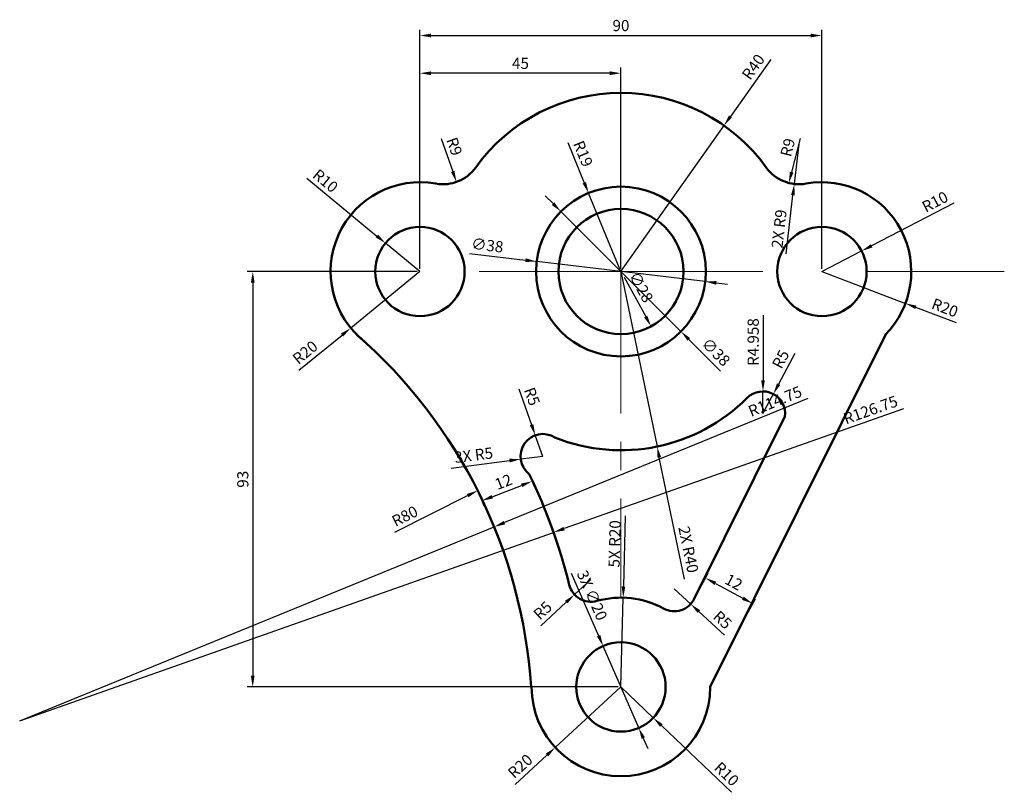
# Model space of a CAD drawing. Units: millimetres. Extents: x -135 to 86, y -117 to 56.
import ezdxf

# ---------------------------------------------------------------- set-up
doc = ezdxf.new("R2010")
doc.units = ezdxf.units.MM
doc.linetypes.add('CENTER', pattern=[50.8, 31.75, -6.35, 6.35, -6.35])
for name, color, linetype, lineweight in [('M-CNTR', 4, 'CENTER', 18), ('M-DIMS', 2, 'Continuous', 25), ('M-OUTL', 7, 'Continuous', 50)]:
    doc.layers.add(name, color=color, linetype=linetype, lineweight=lineweight)
doc.styles.get("Standard").update_dxf_attribs({"font": 'arial.ttf'})
doc.dimstyles.new('ISO-25', dxfattribs={"dimtxt": 2.5, "dimasz": 2.5, "dimexe": 1.25, "dimexo": 0.625, "dimtad": 1, "dimtxsty": 'Standard', "dimcen": 2.5, "dimadec": 0, "dimazin": 0, "dimtfac": 1, "dimtmove": 0, "dimatfit": 3, "dimfxl": 1, "dimarcsym": 0})

# ---------------------------------------------------------------- blocks, each defined once
blk = doc.blocks.new('*D1')
at = {"layer": 'Defpoints', "color": 0, "transparency": 16777216}
for p in [(0, -93), (-14.72, -106.54)]:
    blk.add_point(p, dxfattribs=at)
at = {"layer": 'M-DIMS', "color": 0, "lineweight": -2, "transparency": 16777216}
for p, q in [((0, -93), (-14.72, -106.54)), ((-23.71, -114.81), (-16.56, -108.23))]:
    blk.add_line(p, q, dxfattribs=at)
at = {"layer": 'M-DIMS', "color": 0, "transparency": 16777216}
blk.add_solid([(-16.84, -107.92), (-16.28, -108.54), (-14.72, -106.54)], dxfattribs=at)
at = {"layer": 'M-DIMS', "color": 0, "transparency": 16777216, "insert": (-22.34, -110.96), "char_height": 2.5, "attachment_point": 5, "rotation": 42.6003}
blk.add_mtext('R20', dxfattribs=at)
blk = doc.blocks.new('*D2')
at = {"layer": 'Defpoints', "color": 0, "transparency": 16777216}
for p in [(45, 0), (63.69, -7.12)]:
    blk.add_point(p, dxfattribs=at)
at = {"layer": 'M-DIMS', "color": 0, "lineweight": -2, "transparency": 16777216}
for p, q in [((45, 0), (63.69, -7.12)), ((75.1, -11.48), (66.02, -8.02))]:
    blk.add_line(p, q, dxfattribs=at)
at = {"layer": 'M-DIMS', "color": 0, "transparency": 16777216}
blk.add_solid([(66.17, -7.63), (65.88, -8.4), (63.69, -7.12)], dxfattribs=at)
at = {"layer": 'M-DIMS', "color": 0, "transparency": 16777216, "insert": (72.41, -8.41), "char_height": 2.5, "attachment_point": 5, "rotation": 339.13}
blk.add_mtext('R20', dxfattribs=at)
blk = doc.blocks.new('*D3')
at = {"layer": 'Defpoints', "color": 0, "transparency": 16777216}
for p in [(-45, 0), (-60.5, -12.64)]:
    blk.add_point(p, dxfattribs=at)
at = {"layer": 'M-DIMS', "color": 0, "lineweight": -2, "transparency": 16777216}
for p, q in [((-45, 0), (-60.5, -12.64)), ((-72.11, -22.1), (-62.44, -14.22))]:
    blk.add_line(p, q, dxfattribs=at)
at = {"layer": 'M-DIMS', "color": 0, "transparency": 16777216}
blk.add_solid([(-62.7, -13.89), (-62.18, -14.54), (-60.5, -12.64)], dxfattribs=at)
at = {"layer": 'M-DIMS', "color": 0, "transparency": 16777216, "insert": (-70.51, -18.35), "char_height": 2.5, "attachment_point": 5, "rotation": 39.1885}
blk.add_mtext('R20', dxfattribs=at)
blk = doc.blocks.new('*D4')
at = {"layer": 'Defpoints', "color": 0, "transparency": 16777216}
for p in [(-52.72, 6.36), (-45, 0)]:
    blk.add_point(p, dxfattribs=at)
at = {"layer": 'M-DIMS', "color": 0, "lineweight": -2, "transparency": 16777216}
for p, q in [((-70.35, 20.88), (-54.65, 7.95)), ((-45, 0), (-52.72, 6.36))]:
    blk.add_line(p, q, dxfattribs=at)
at = {"layer": 'M-DIMS', "color": 0, "transparency": 16777216}
blk.add_solid([(-54.38, 8.27), (-54.91, 7.63), (-52.72, 6.36)], dxfattribs=at)
at = {"layer": 'M-DIMS', "color": 0, "transparency": 16777216, "insert": (-66.36, 20.05), "char_height": 2.5, "attachment_point": 5, "rotation": 320.5239}
blk.add_mtext('R10', dxfattribs=at)
blk = doc.blocks.new('*D5')
at = {"layer": 'Defpoints', "color": 0, "transparency": 16777216}
for p in [(53.88, 4.6), (45, 0)]:
    blk.add_point(p, dxfattribs=at)
at = {"layer": 'M-DIMS', "color": 0, "lineweight": -2, "transparency": 16777216}
for p, q in [((74.53, 15.3), (56.1, 5.75)), ((45, 0), (53.88, 4.6))]:
    blk.add_line(p, q, dxfattribs=at)
at = {"layer": 'M-DIMS', "color": 0, "transparency": 16777216}
blk.add_solid([(55.91, 6.12), (56.29, 5.38), (53.88, 4.6)], dxfattribs=at)
at = {"layer": 'M-DIMS', "color": 0, "transparency": 16777216, "insert": (70.46, 15.33), "char_height": 2.5, "attachment_point": 5, "rotation": 27.3837}
blk.add_mtext('R10', dxfattribs=at)
blk = doc.blocks.new('*D6')
at = {"layer": 'Defpoints', "color": 0, "transparency": 16777216}
for p in [(0, -93), (7.24, -99.9)]:
    blk.add_point(p, dxfattribs=at)
at = {"layer": 'M-DIMS', "color": 0, "lineweight": -2, "transparency": 16777216}
for p, q in [((0, -93), (7.24, -99.9)), ((24.73, -116.58), (9.05, -101.63))]:
    blk.add_line(p, q, dxfattribs=at)
at = {"layer": 'M-DIMS', "color": 0, "transparency": 16777216}
blk.add_solid([(9.33, -101.32), (8.76, -101.93), (7.24, -99.9)], dxfattribs=at)
at = {"layer": 'M-DIMS', "color": 0, "transparency": 16777216, "insert": (23.43, -112.71), "char_height": 2.5, "attachment_point": 5, "rotation": 316.3688}
blk.add_mtext('R10', dxfattribs=at)
blk = doc.blocks.new('*D7')
at = {"layer": 'Defpoints', "color": 0, "transparency": 16777216}
for p in [(23.07, 32.68), (0, 0)]:
    blk.add_point(p, dxfattribs=at)
at = {"layer": 'M-DIMS', "color": 0, "lineweight": -2, "transparency": 16777216}
for p, q in [((33.52, 47.48), (24.51, 34.72)), ((0, 0), (23.07, 32.68))]:
    blk.add_line(p, q, dxfattribs=at)
at = {"layer": 'M-DIMS', "color": 0, "transparency": 16777216}
blk.add_solid([(24.17, 34.96), (24.85, 34.48), (23.07, 32.68)], dxfattribs=at)
at = {"layer": 'M-DIMS', "color": 0, "transparency": 16777216, "insert": (29.89, 45.63), "char_height": 2.5, "attachment_point": 5, "rotation": 54.7774}
blk.add_mtext('R40', dxfattribs=at)
blk = doc.blocks.new('*D8')
at = {"layer": 'Defpoints', "color": 0, "transparency": 16777216}
for p in [(-6.74, 12.27), (6.74, -12.27)]:
    blk.add_point(p, dxfattribs=at)
at = {"layer": 'M-DIMS', "color": 0, "lineweight": -2, "transparency": 16777216}
blk.add_line((0.7, -1.27), (5.54, -10.08), dxfattribs=at)
at = {"layer": 'M-DIMS', "color": 0, "transparency": 16777216}
blk.add_solid([(5.9, -9.88), (5.17, -10.28), (6.74, -12.27)], dxfattribs=at)
at = {"layer": 'M-DIMS', "color": 0, "transparency": 16777216, "insert": (4.24, -3.63), "char_height": 2.5, "attachment_point": 5, "rotation": 298.7887}
blk.add_mtext('∅28', dxfattribs=at)
blk = doc.blocks.new('*D9')
at = {"layer": 'Defpoints', "color": 0, "transparency": 16777216}
for p in [(-13.44, 13.43), (13.44, -13.43)]:
    blk.add_point(p, dxfattribs=at)
at = {"layer": 'M-DIMS', "color": 0, "lineweight": -2, "transparency": 16777216}
for p, q in [((-15.21, 15.2), (-16.98, 16.96)), ((-13.44, 13.43), (13.44, -13.43)), ((22.32, -22.3), (15.21, -15.2))]:
    blk.add_line(p, q, dxfattribs=at)
at = {"layer": 'M-DIMS', "color": 0, "transparency": 16777216}
for points in [[(-14.92, 15.49), (-15.5, 14.9), (-13.44, 13.43)], [(15.5, -14.9), (14.92, -15.49), (13.44, -13.43)]]:
    blk.add_solid(points, dxfattribs=at)
at = {"layer": 'M-DIMS', "color": 0, "transparency": 16777216, "insert": (21.04, -18.24), "char_height": 2.5, "attachment_point": 5, "rotation": 315.0277}
blk.add_mtext('∅38', dxfattribs=at)
blk = doc.blocks.new('*D10')
at = {"layer": 'Defpoints', "color": 0, "transparency": 16777216}
for p in [(39.83, 28.54), (37.59, 19.82)]:
    blk.add_point(p, dxfattribs=at)
at = {"layer": 'M-DIMS', "color": 0, "lineweight": -2, "transparency": 16777216}
blk.add_line((40.15, 29.78), (38.21, 22.24), dxfattribs=at)
at = {"layer": 'M-DIMS', "color": 0, "transparency": 16777216}
blk.add_solid([(37.81, 22.35), (38.62, 22.14), (37.59, 19.82)], dxfattribs=at)
at = {"layer": 'M-DIMS', "color": 0, "transparency": 16777216, "insert": (37.65, 27.7), "char_height": 2.5, "attachment_point": 5, "rotation": 75.5659}
blk.add_mtext('R9', dxfattribs=at)
blk = doc.blocks.new('*D11')
at = {"layer": 'Defpoints', "color": 0, "transparency": 16777216}
for p in [(-39.83, 28.54), (-36.84, 20.05)]:
    blk.add_point(p, dxfattribs=at)
at = {"layer": 'M-DIMS', "color": 0, "lineweight": -2, "transparency": 16777216}
blk.add_line((-40.26, 29.75), (-37.67, 22.41), dxfattribs=at)
at = {"layer": 'M-DIMS', "color": 0, "transparency": 16777216}
blk.add_solid([(-37.28, 22.55), (-38.06, 22.27), (-36.84, 20.05)], dxfattribs=at)
at = {"layer": 'M-DIMS', "color": 0, "transparency": 16777216, "insert": (-37.59, 27.89), "char_height": 2.5, "attachment_point": 5, "rotation": 289.4447}
blk.add_mtext('R9', dxfattribs=at)
blk = doc.blocks.new('*D12')
at = {"layer": 'Defpoints', "color": 0, "transparency": 16777216}
for p in [(-7.25, 17.56), (0, 0)]:
    blk.add_point(p, dxfattribs=at)
at = {"layer": 'M-DIMS', "color": 0, "lineweight": -2, "transparency": 16777216}
for p, q in [((-11.91, 28.87), (-8.2, 19.87)), ((0, 0), (-7.25, 17.56))]:
    blk.add_line(p, q, dxfattribs=at)
at = {"layer": 'M-DIMS', "color": 0, "transparency": 16777216}
blk.add_solid([(-7.82, 20.03), (-8.59, 19.72), (-7.25, 17.56)], dxfattribs=at)
at = {"layer": 'M-DIMS', "color": 0, "transparency": 16777216, "insert": (-8.78, 26.25), "char_height": 2.5, "attachment_point": 5, "rotation": 292.423}
blk.add_mtext('R19', dxfattribs=at)
blk = doc.blocks.new('*D13')
at = {"layer": 'Defpoints', "color": 0, "transparency": 16777216}
for p in [(-45, 44.39), (0, 0), (-45, 0)]:
    blk.add_point(p, dxfattribs=at)
at = {"layer": 'M-DIMS', "color": 0, "lineweight": -2, "transparency": 16777216}
for p, q in [((-45, 0.62), (-45, 45.64)), ((-2.5, 44.39), (-42.5, 44.39)), ((0, 0.62), (0, 45.64))]:
    blk.add_line(p, q, dxfattribs=at)
at = {"layer": 'M-DIMS', "color": 0, "transparency": 16777216}
for points in [[(-42.5, 44.81), (-42.5, 43.97), (-45, 44.39)], [(-2.5, 44.81), (-2.5, 43.97), (0, 44.39)]]:
    blk.add_solid(points, dxfattribs=at)
at = {"layer": 'M-DIMS', "color": 0, "transparency": 16777216, "insert": (-22.5, 46.29), "char_height": 2.5, "attachment_point": 5}
blk.add_mtext('45', dxfattribs=at)
blk = doc.blocks.new('*D14')
at = {"layer": 'Defpoints', "color": 0, "transparency": 16777216}
for p in [(45, 52.83), (45, 0), (-45, 0)]:
    blk.add_point(p, dxfattribs=at)
at = {"layer": 'M-DIMS', "color": 0, "lineweight": -2, "transparency": 16777216}
for p, q in [((-45, 0.62), (-45, 54.08)), ((45, 0.62), (45, 54.08)), ((-42.5, 52.83), (42.5, 52.83))]:
    blk.add_line(p, q, dxfattribs=at)
at = {"layer": 'M-DIMS', "color": 0, "transparency": 16777216}
for points in [[(-42.5, 53.25), (-42.5, 52.42), (-45, 52.83)], [(42.5, 53.25), (42.5, 52.42), (45, 52.83)]]:
    blk.add_solid(points, dxfattribs=at)
at = {"layer": 'M-DIMS', "color": 0, "transparency": 16777216, "insert": (0, 54.74), "char_height": 2.5, "attachment_point": 5}
blk.add_mtext('90', dxfattribs=at)
blk = doc.blocks.new('*D15')
at = {"layer": 'Defpoints', "color": 0, "transparency": 16777216}
for p in [(16.41, -73.26), (29.49, -74.33), (26.97, -78.98)]:
    blk.add_point(p, dxfattribs=at)
at = {"layer": 'M-DIMS', "color": 0, "lineweight": -2, "transparency": 16777216}
for p, q in [((16.71, -72.71), (19.53, -67.51)), ((21.13, -69.8), (27.29, -73.13)), ((27.27, -78.43), (30.09, -73.23))]:
    blk.add_line(p, q, dxfattribs=at)
at = {"layer": 'M-DIMS', "color": 0, "transparency": 16777216}
for points in [[(21.33, -69.43), (20.93, -70.17), (18.93, -68.61)], [(27.49, -72.77), (27.1, -73.5), (29.49, -74.33)]]:
    blk.add_solid(points, dxfattribs=at)
at = {"layer": 'M-DIMS', "color": 0, "transparency": 16777216, "insert": (25.11, -69.81), "char_height": 2.5, "attachment_point": 5, "rotation": 331.5726}
blk.add_mtext('12', dxfattribs=at)
blk = doc.blocks.new('*D16')
at = {"layer": 'Defpoints', "color": 0, "transparency": 16777216}
for p in [(-20.54, -45.33), (-19.9, -46.96), (-31.77, -49.68)]:
    blk.add_point(p, dxfattribs=at)
at = {"layer": 'M-DIMS', "color": 0, "lineweight": -2, "transparency": 16777216}
for p, q in [((-20.31, -45.92), (-19.45, -48.13)), ((-28.81, -50.41), (-22.24, -47.87)), ((-31.54, -50.26), (-30.69, -52.48))]:
    blk.add_line(p, q, dxfattribs=at)
at = {"layer": 'M-DIMS', "color": 0, "transparency": 16777216}
for points in [[(-22.39, -47.48), (-22.09, -48.25), (-19.9, -46.96)], [(-28.96, -50.02), (-28.66, -50.8), (-31.14, -51.31)]]:
    blk.add_solid(points, dxfattribs=at)
at = {"layer": 'M-DIMS', "color": 0, "transparency": 16777216, "insert": (-26.2, -47.38), "char_height": 2.5, "attachment_point": 5, "rotation": 21.1544}
blk.add_mtext('12', dxfattribs=at)
blk = doc.blocks.new('*D17')
at = {"layer": 'Defpoints', "color": 0, "transparency": 16777216}
for p in [(-32.09, -49.04), (-134.61, -100.59)]:
    blk.add_point(p, dxfattribs=at)
at = {"layer": 'M-DIMS', "color": 0, "lineweight": -2, "transparency": 16777216}
blk.add_line((-50.61, -58.36), (-34.32, -50.17), dxfattribs=at)
at = {"layer": 'M-DIMS', "color": 0, "transparency": 16777216}
blk.add_solid([(-34.51, -49.79), (-34.13, -50.54), (-32.09, -49.04)], dxfattribs=at)
at = {"layer": 'M-DIMS', "color": 0, "transparency": 16777216, "insert": (-48.24, -55.04), "char_height": 2.5, "attachment_point": 5, "rotation": 26.6892}
blk.add_mtext('R80', dxfattribs=at)
blk = doc.blocks.new('*D18')
at = {"layer": 'Defpoints', "color": 0, "transparency": 16777216}
for p in [(-45, 0), (-82.44, -93), (0, -93)]:
    blk.add_point(p, dxfattribs=at)
at = {"layer": 'M-DIMS', "color": 0, "lineweight": -2, "transparency": 16777216}
for p, q in [((-45.63, 0), (-83.69, 0)), ((-82.44, -2.5), (-82.44, -90.5)), ((-0.63, -93), (-83.69, -93))]:
    blk.add_line(p, q, dxfattribs=at)
at = {"layer": 'M-DIMS', "color": 0, "transparency": 16777216}
for points in [[(-82.85, -2.5), (-82.02, -2.5), (-82.44, 0)], [(-82.85, -90.5), (-82.02, -90.5), (-82.44, -93)]]:
    blk.add_solid(points, dxfattribs=at)
at = {"layer": 'M-DIMS', "color": 0, "transparency": 16777216, "insert": (-84.34, -46.5), "char_height": 2.5, "attachment_point": 5, "rotation": 90}
blk.add_mtext('93', dxfattribs=at)
blk = doc.blocks.new('*D19')
at = {"layer": 'Defpoints', "color": 0, "transparency": 16777216}
for p in [(-19.17, -36.66), (-17.49, -41.37)]:
    blk.add_point(p, dxfattribs=at)
at = {"layer": 'M-DIMS', "color": 0, "lineweight": -2, "transparency": 16777216}
for p, q in [((-22.89, -26.22), (-20.01, -34.3)), ((-17.49, -41.37), (-19.17, -36.66))]:
    blk.add_line(p, q, dxfattribs=at)
at = {"layer": 'M-DIMS', "color": 0, "transparency": 16777216}
blk.add_solid([(-19.62, -34.16), (-20.4, -34.44), (-19.17, -36.66)], dxfattribs=at)
at = {"layer": 'M-DIMS', "color": 0, "transparency": 16777216, "insert": (-20.21, -28.08), "char_height": 2.5, "attachment_point": 5, "rotation": 289.6107}
blk.add_mtext('R5', dxfattribs=at)
blk = doc.blocks.new('*D20')
at = {"layer": 'Defpoints', "color": 0, "transparency": 16777216}
for p in [(34.12, -27.41), (31.79, -31.79)]:
    blk.add_point(p, dxfattribs=at)
at = {"layer": 'M-DIMS', "color": 0, "lineweight": -2, "transparency": 16777216}
for p, q in [((38.96, -18.32), (35.29, -25.21)), ((31.79, -31.79), (34.12, -27.41))]:
    blk.add_line(p, q, dxfattribs=at)
at = {"layer": 'M-DIMS', "color": 0, "transparency": 16777216}
blk.add_solid([(34.93, -25.01), (35.66, -25.4), (34.12, -27.41)], dxfattribs=at)
at = {"layer": 'M-DIMS', "color": 0, "transparency": 16777216, "insert": (36.04, -19.77), "char_height": 2.5, "attachment_point": 5, "rotation": 61.9797}
blk.add_mtext('R5', dxfattribs=at)
blk = doc.blocks.new('*D21')
at = {"layer": 'Defpoints', "color": 0, "transparency": 16777216}
for p in [(11.94, -71.03), (15.61, -74.43)]:
    blk.add_point(p, dxfattribs=at)
at = {"layer": 'M-DIMS', "color": 0, "lineweight": -2, "transparency": 16777216}
for p, q in [((11.94, -71.03), (15.61, -74.43)), ((23.18, -81.41), (17.45, -76.12))]:
    blk.add_line(p, q, dxfattribs=at)
at = {"layer": 'M-DIMS', "color": 0, "transparency": 16777216}
blk.add_solid([(17.73, -75.82), (17.17, -76.43), (15.61, -74.43)], dxfattribs=at)
at = {"layer": 'M-DIMS', "color": 0, "transparency": 16777216, "insert": (22.52, -78.22), "char_height": 2.5, "attachment_point": 5, "rotation": 317.2922}
blk.add_mtext('R5', dxfattribs=at)
blk = doc.blocks.new('*D22')
at = {"layer": 'Defpoints', "color": 0, "transparency": 16777216}
for p in [(-6.72, -68.92), (-10.4, -72.31)]:
    blk.add_point(p, dxfattribs=at)
at = {"layer": 'M-DIMS', "color": 0, "lineweight": -2, "transparency": 16777216}
for p, q in [((-6.72, -68.92), (-10.4, -72.31)), ((-17.96, -79.3), (-12.23, -74.01))]:
    blk.add_line(p, q, dxfattribs=at)
at = {"layer": 'M-DIMS', "color": 0, "transparency": 16777216}
blk.add_solid([(-12.51, -73.7), (-11.95, -74.31), (-10.4, -72.31)], dxfattribs=at)
at = {"layer": 'M-DIMS', "color": 0, "transparency": 16777216, "insert": (-17.3, -76.11), "char_height": 2.5, "attachment_point": 5, "rotation": 42.7122}
blk.add_mtext('R5', dxfattribs=at)
blk = doc.blocks.new('MOUNTING-HOLE-D20')
blk.add_circle((10, 10), 10)
blk = doc.blocks.new('*D24')
at = {"layer": 'Defpoints', "color": 0, "transparency": 16777216}
for p in [(0, 0), (8.09, -39.17)]:
    blk.add_point(p, dxfattribs=at)
at = {"layer": 'M-DIMS', "color": 0, "lineweight": -2, "transparency": 16777216}
for p, q in [((0, 0), (8.09, -39.17)), ((14.22, -68.86), (8.59, -41.62))]:
    blk.add_line(p, q, dxfattribs=at)
at = {"layer": 'M-DIMS', "color": 0, "transparency": 16777216}
blk.add_solid([(9, -41.54), (8.19, -41.71), (8.09, -39.17)], dxfattribs=at)
at = {"layer": 'M-DIMS', "color": 0, "transparency": 16777216, "insert": (14.8, -62.29), "char_height": 2.5, "attachment_point": 5, "rotation": 281.6656}
blk.add_mtext('2X R40', dxfattribs=at)
blk = doc.blocks.new('*D25')
at = {"layer": 'Defpoints', "color": 0, "transparency": 16777216}
for p in [(-18.87, 2.25), (18.87, -2.25)]:
    blk.add_point(p, dxfattribs=at)
at = {"layer": 'M-DIMS', "color": 0, "lineweight": -2, "transparency": 16777216}
for p, q in [((-33.94, 4.05), (-21.35, 2.55)), ((18.87, -2.25), (-18.87, 2.25)), ((21.35, -2.55), (23.83, -2.84))]:
    blk.add_line(p, q, dxfattribs=at)
at = {"layer": 'M-DIMS', "color": 0, "transparency": 16777216}
for points in [[(-21.3, 2.96), (-21.4, 2.13), (-18.87, 2.25)], [(21.4, -2.13), (21.3, -2.96), (18.87, -2.25)]]:
    blk.add_solid(points, dxfattribs=at)
at = {"layer": 'M-DIMS', "color": 0, "transparency": 16777216, "insert": (-29.95, 5.56), "char_height": 2.5, "attachment_point": 5, "rotation": 353.2003}
blk.add_mtext('∅38', dxfattribs=at)
blk = doc.blocks.new('*D26')
at = {"layer": 'Defpoints', "color": 0, "transparency": 16777216}
for p in [(-4, -83.83), (4, -102.17)]:
    blk.add_point(p, dxfattribs=at)
at = {"layer": 'M-DIMS', "color": 0, "lineweight": -2, "transparency": 16777216}
for p, q in [((-11.11, -67.54), (-5, -81.54)), ((4, -102.17), (-4, -83.83)), ((5, -104.46), (6, -106.75))]:
    blk.add_line(p, q, dxfattribs=at)
at = {"layer": 'M-DIMS', "color": 0, "transparency": 16777216}
for points in [[(-4.62, -81.38), (-5.38, -81.71), (-4, -83.83)], [(5.38, -104.29), (4.62, -104.62), (4, -102.17)]]:
    blk.add_solid(points, dxfattribs=at)
at = {"layer": 'M-DIMS', "color": 0, "transparency": 16777216, "insert": (-6.75, -72.61), "char_height": 2.5, "attachment_point": 5, "rotation": 293.5785}
blk.add_mtext('3X ∅20', dxfattribs=at)
blk = doc.blocks.new('*D27')
at = {"layer": 'Defpoints', "color": 0, "transparency": 16777216}
for p in [(0.5, -73.01), (0, -93)]:
    blk.add_point(p, dxfattribs=at)
at = {"layer": 'M-DIMS', "color": 0, "lineweight": -2, "transparency": 16777216}
for p, q in [((0.96, -54.72), (0.56, -70.51)), ((0, -93), (0.5, -73.01))]:
    blk.add_line(p, q, dxfattribs=at)
at = {"layer": 'M-DIMS', "color": 0, "transparency": 16777216}
blk.add_solid([(0.15, -70.5), (0.98, -70.52), (0.5, -73.01)], dxfattribs=at)
at = {"layer": 'M-DIMS', "color": 0, "transparency": 16777216, "insert": (-1.1, -60.96), "char_height": 2.5, "attachment_point": 5, "rotation": 88.5675}
blk.add_mtext('5X R20', dxfattribs=at)
blk = doc.blocks.new('*D28')
at = {"layer": 'Defpoints', "color": 0, "transparency": 16777216}
for p in [(39.83, 28.54), (38.8, 19.6)]:
    blk.add_point(p, dxfattribs=at)
at = {"layer": 'M-DIMS', "color": 0, "lineweight": -2, "transparency": 16777216}
for p, q in [((39.83, 28.54), (38.8, 19.6)), ((37, 4), (38.51, 17.11))]:
    blk.add_line(p, q, dxfattribs=at)
at = {"layer": 'M-DIMS', "color": 0, "transparency": 16777216}
blk.add_solid([(38.1, 17.16), (38.93, 17.06), (38.8, 19.6)], dxfattribs=at)
at = {"layer": 'M-DIMS', "color": 0, "transparency": 16777216, "insert": (35.72, 9.53), "char_height": 2.5, "attachment_point": 5, "rotation": 83.4038}
blk.add_mtext('2X R9', dxfattribs=at)
blk = doc.blocks.new('*D29')
at = {"layer": 'Defpoints', "color": 0, "transparency": 16777216}
for p in [(-17.49, -41.37), (-22.45, -42)]:
    blk.add_point(p, dxfattribs=at)
at = {"layer": 'M-DIMS', "color": 0, "lineweight": -2, "transparency": 16777216}
for p, q in [((-17.49, -41.37), (-22.45, -42)), ((-38, -43.98), (-24.93, -42.32))]:
    blk.add_line(p, q, dxfattribs=at)
at = {"layer": 'M-DIMS', "color": 0, "transparency": 16777216}
blk.add_solid([(-24.98, -41.9), (-24.88, -42.73), (-22.45, -42)], dxfattribs=at)
at = {"layer": 'M-DIMS', "color": 0, "transparency": 16777216, "insert": (-32.94, -41.42), "char_height": 2.5, "attachment_point": 5, "rotation": 7.2718}
blk.add_mtext('3X R5', dxfattribs=at)
blk = doc.blocks.new('*D30')
at = {"layer": 'Defpoints', "color": 0, "transparency": 16777216}
for p in [(31.8, -26.83), (31.79, -31.79)]:
    blk.add_point(p, dxfattribs=at)
at = {"layer": 'M-DIMS', "color": 0, "lineweight": -2, "transparency": 16777216}
for p, q in [((31.83, -9.75), (31.81, -24.33)), ((31.79, -31.79), (31.8, -26.83))]:
    blk.add_line(p, q, dxfattribs=at)
at = {"layer": 'M-DIMS', "color": 0, "transparency": 16777216}
blk.add_solid([(31.39, -24.33), (32.22, -24.33), (31.8, -26.83)], dxfattribs=at)
at = {"layer": 'M-DIMS', "color": 0, "transparency": 16777216, "insert": (29.92, -15.79), "char_height": 2.5, "attachment_point": 5, "rotation": 89.8848}
blk.add_mtext('R4.958', dxfattribs=at)
blk = doc.blocks.new('*D31')
at = {"layer": 'Defpoints', "color": 0, "transparency": 16777216}
for p in [(-28.39, -57.16), (-134.61, -100.59)]:
    blk.add_point(p, dxfattribs=at)
at = {"layer": 'M-DIMS', "color": 0, "lineweight": -2, "transparency": 16777216}
for p, q in [((41.84, -28.45), (-26.08, -56.21)), ((-134.61, -100.59), (-28.39, -57.16))]:
    blk.add_line(p, q, dxfattribs=at)
at = {"layer": 'M-DIMS', "color": 0, "transparency": 16777216}
blk.add_solid([(-26.24, -55.83), (-25.92, -56.6), (-28.39, -57.16)], dxfattribs=at)
at = {"layer": 'M-DIMS', "color": 0, "transparency": 16777216, "insert": (34.62, -29.35), "char_height": 2.5, "attachment_point": 5, "rotation": 22.2357}
blk.add_mtext('R114.75', dxfattribs=at)
blk = doc.blocks.new('*D32')
at = {"layer": 'Defpoints', "color": 0, "transparency": 16777216}
for p in [(-15.09, -58.39), (-134.61, -100.59)]:
    blk.add_point(p, dxfattribs=at)
at = {"layer": 'M-DIMS', "color": 0, "lineweight": -2, "transparency": 16777216}
for p, q in [((63.24, -30.73), (-12.73, -57.55)), ((-134.61, -100.59), (-15.09, -58.39))]:
    blk.add_line(p, q, dxfattribs=at)
at = {"layer": 'M-DIMS', "color": 0, "transparency": 16777216}
blk.add_solid([(-12.87, -57.16), (-12.59, -57.95), (-15.09, -58.39)], dxfattribs=at)
at = {"layer": 'M-DIMS', "color": 0, "transparency": 16777216, "insert": (55.99, -31.27), "char_height": 2.5, "attachment_point": 5, "rotation": 19.4469}
blk.add_mtext('R126.75', dxfattribs=at)

msp = doc.modelspace()

# ---------------------------------------------------------------- linework, layer by layer
at = {"layer": 'M-CNTR'}
for p, q in [((0, 0), (-35, 0)), ((0, 0), (35, 0)), ((0, 0), (0, -73)), ((55, 0), (85.8249, 0))]:
    msp.add_line(p, q, dxfattribs=at)
at = {"layer": 'M-OUTL'}
for p, q in [((59.2952, -13.9874), (20, -93)), ((36.7011, -32.4702), (16.4147, -73.2609)), ((-20, -93), (-20.1107, -93))]:
    msp.add_line(p, q, dxfattribs=at)
for radius in [19, 14]:
    msp.add_circle((0, 0), radius, dxfattribs=at)
for centre, radius, start, end in [((0, 0), 40, 35.617279, 144.382721), ((-39.8333, 28.536), 9, 259.737343, 324.382721), ((39.8333, 28.536), 9, 215.617279, 280.262657), ((-45, 0), 20, 79.737343, 231.603886), ((45, 0), 20, 315, 100.262657), ((-134.6119, -100.5851), 114.7522, 3.789988, 48.877125), ((0, 0), 40, 248.330038, 315), ((31.79, -31.79), 4.9579, 352.115083, 135), ((-17.4921, -41.3674), 5, 57.02018, 232.512106), ((-134.6119, -100.5851), 126.7522, 13.906281, 25.84208), ((-6.7213, -68.9205), 5, 193.906281, 285.596079), ((0, -93), 20, 61.476926, 105.596079), ((0, -93), 20, 61.476926, 105.596079), ((11.9378, -71.0344), 5, 241.476926, 333.557542), ((0, -93), 20, 180, 360)]:
    msp.add_arc(centre, radius, start, end, dxfattribs=at)

# ---------------------------------------------------------------- block references
for p in [(-55, -10), (35, -10), (-10, -103)]:
    msp.add_blockref('MOUNTING-HOLE-D20', p, dxfattribs=at)

# ---------------------------------------------------------------- dimensions: what is measured, and where the dimension line sits
at = {"layer": 'M-DIMS'}
for base, p1, p2, picture, middle in [((45, 52.8349), (-45, 0), (45, 0), '*D14', (0, 54.7363)), ((-45, 44.3906), (0, 0), (-45, 0), '*D13', (-22.5, 46.2869))]:
    dim = msp.add_linear_dim(base=base, p1=p1, p2=p2, dimstyle='ISO-25', override={"dimclrd": 0, "dimclre": 0, "dimclrt": 0}, dxfattribs=at)
    dim.commit()
    dim.dimension.update_dxf_attribs({"geometry": picture, "text_midpoint": middle})
for center, mpoint, override, picture, middle in [((0, 0), (23.0702, 32.6767), {"dimclrd": 0, "dimclre": 0, "dimclrt": 0}, '*D7', (31.4396, 44.5312)), ((-39.8333, 28.536), (-36.8373, 20.0494), {"dimclrd": 0, "dimclre": 0, "dimclrt": 0}, '*D11', (-39.3817, 27.2567)), ((39.8333, 28.536), (37.5899, 19.8201), {"dimclrd": 0, "dimclre": 0, "dimclrt": 0}, '*D10', (39.4951, 27.2221)), ((-45, 0), (-52.7189, 6.3576), {"dimclrd": 0, "dimclre": 0, "dimclrt": 0}, '*D4', (-67.5648, 18.5852)), ((45, 0), (53.8795, 4.5995), {"dimclrd": 0, "dimclre": 0, "dimclrt": 0}, '*D5', (71.3306, 13.639)), ((-45, 0), (-60.5014, -12.6375), {"dimclrd": 0, "dimclre": 0, "dimclrt": 0}, '*D3', (-69.3119, -19.8202)), ((-134.6119, -100.5851), (-28.3933, -57.1608), {"dimdec": 2, "dimlfac": 1, "dimrnd": 0, "dimzin": 0, "dimdsep": 46, "dimlunit": 2}, '*D31', (35.3379, -31.1062)), ((-17.4921, -41.3674), (-19.1702, -36.6574), {"dimclrd": 0, "dimclre": 0, "dimclrt": 0}, '*D19', (-21.9992, -28.7175)), ((-134.6119, -100.5851), (-15.0908, -58.3851), {"dimdec": 2, "dimlfac": 1, "dimrnd": 0, "dimzin": 0, "dimdsep": 46, "dimlunit": 2}, '*D32', (56.6218, -33.0652)), ((0, -93), (7.238, -99.9001), {"dimclrd": 0, "dimclre": 0, "dimclrt": 0}, '*D6', (22.1203, -114.0879))]:
    dim = msp.add_radius_dim(center=center, mpoint=mpoint, dimstyle='ISO-25', override=override, dxfattribs=at)
    dim.commit()
    dim.dimension.update_dxf_attribs({"geometry": picture, "text_midpoint": middle, "dimtype": 164})
for center, mpoint, override, picture, middle in [((0, 0), (-7.2474, 17.5635), {"dimclrd": 0, "dimclre": 0, "dimclrt": 0}, '*D12', (-8.7756, 26.2519)), ((45, 0), (63.6878, -7.125), {"dimclrd": 0, "dimclre": 0, "dimclrt": 0}, '*D2', (72.4081, -8.4148)), ((31.79, -31.79), (31.8, -26.8321), {"dimdec": 3, "dimlfac": 1, "dimrnd": 0, "dimzin": 0, "dimdsep": 46, "dimlunit": 2}, '*D30', (29.9208, -15.7864)), ((-6.7213, -68.9205), (-10.3952, -72.3121), {"dimclrd": 0, "dimclre": 0, "dimclrt": 0}, '*D22', (-17.3025, -76.1079)), ((11.9378, -71.0344), (15.6119, -74.4257), {"dimclrd": 0, "dimclre": 0, "dimclrt": 0}, '*D21', (22.5196, -78.221)), ((0, -93), (-14.7219, -106.5376), {"dimclrd": 0, "dimclre": 0, "dimclrt": 0}, '*D1', (-22.3449, -110.9643))]:
    dim = msp.add_radius_dim(center=center, mpoint=mpoint, dimstyle='ISO-25', override=override, dxfattribs=at)
    dim.commit()
    dim.dimension.update_dxf_attribs({"geometry": picture, "text_midpoint": middle})
for center, mpoint, text, override, picture, middle in [((39.8333, 28.536), (38.7995, 19.5956), '2X <>', {"dimdec": 0, "dimlfac": 1, "dimrnd": 0, "dimzin": 0, "dimdsep": 46, "dimlunit": 2}, '*D28', (35.7217, 9.5321)), ((31.79, -31.79), (34.1192, -27.4133), 'R5', {"dimclrd": 0, "dimclre": 0, "dimclrt": 0}, '*D20', (36.0391, -19.7691)), ((-17.4921, -41.3674), (-22.4519, -42.0002), '3X <>', {"dimdec": 0, "dimlfac": 1, "dimrnd": 0, "dimzin": 0, "dimdsep": 46, "dimlunit": 2}, '*D29', (-32.9446, -41.4214))]:
    dim = msp.add_radius_dim(center=center, mpoint=mpoint, text=text, dimstyle='ISO-25', override=override, dxfattribs=at)
    dim.commit()
    dim.dimension.update_dxf_attribs({"geometry": picture, "text_midpoint": middle})
dim = msp.add_diameter_dim_2p(p1=(-13.4415, 13.4285), p2=(13.4415, -13.4285), dimstyle='ISO-25', override={"dimclrd": 0, "dimclre": 0, "dimclrt": 0}, dxfattribs=at)
dim.commit()
dim.dimension.update_dxf_attribs({"geometry": '*D9', "text_midpoint": (21.0449, -18.238)})
for p1, p2, override, picture, middle in [((-6.7421, 12.2696), (6.7421, -12.2696), {"dimclrd": 0, "dimclre": 0, "dimclrt": 0}, '*D8', (2.5148, -4.5764)), ((18.8664, -2.2496), (-18.8664, 2.2496), {"dimdec": 0, "dimlfac": 1, "dimrnd": 0, "dimzin": 0, "dimdsep": 46, "dimlunit": 2}, '*D25', (-30.1862, 3.5993))]:
    dim = msp.add_diameter_dim_2p(p1=p1, p2=p2, dimstyle='ISO-25', override=override, dxfattribs=at)
    dim.commit()
    dim.dimension.update_dxf_attribs({"geometry": picture, "text_midpoint": middle, "dimtype": 163})
dim = msp.add_linear_dim(base=(-82.4383, -93), p1=(-45, 0), p2=(0, -93), angle=90, dimstyle='ISO-25', override={"dimclrd": 0, "dimclre": 0, "dimclrt": 0}, dxfattribs=at)
dim.commit()
dim.dimension.update_dxf_attribs({"geometry": '*D18', "text_midpoint": (-84.3406, -46.5)})
for center, mpoint, text, override, picture, middle in [((0, 0), (8.088, -39.1738), '2X <>', {"dimdec": 0, "dimlfac": 1, "dimrnd": 0, "dimzin": 0, "dimdsep": 46, "dimlunit": 2}, '*D24', (12.9407, -62.678)), ((-134.6119, -100.5851), (-32.0859, -49.044), 'R80', {"dimclrd": 0, "dimclre": 0, "dimclrt": 0}, '*D17', (-47.3863, -56.7357)), ((0, -93), (0.5, -73.0063), '5X <>', {"dimdec": 0, "dimlfac": 1, "dimrnd": 0, "dimzin": 0, "dimdsep": 46, "dimlunit": 2}, '*D27', (0.8, -61.01))]:
    dim = msp.add_radius_dim(center=center, mpoint=mpoint, text=text, dimstyle='ISO-25', override=override, dxfattribs=at)
    dim.commit()
    dim.dimension.update_dxf_attribs({"geometry": picture, "text_midpoint": middle, "dimtype": 164})
for p1, p2, distance, picture, middle in [((-31.7679, -49.6814), (-20.5351, -45.3348), -1.7463, '*D16', (-26.1998, -47.3833)), ((16.4147, -73.2609), (26.9741, -78.9768), 5.2897, '*D15', (25.1076, -69.8136))]:
    dim = msp.add_aligned_dim(p1=p1, p2=p2, distance=distance, text='12', dimstyle='ISO-25', override={"dimclrd": 0, "dimclre": 0, "dimclrt": 0}, dxfattribs=at)
    dim.commit()
    dim.dimension.update_dxf_attribs({"geometry": picture, "text_midpoint": middle})
dim = msp.add_diameter_dim_2p(p1=(4.0001, -102.1651), p2=(-4.0001, -83.8349), text='3X <>', dimstyle='ISO-25', override={"dimdec": 0, "dimlfac": 1, "dimrnd": 0, "dimzin": 0, "dimdsep": 46, "dimlunit": 2}, dxfattribs=at)
dim.commit()
dim.dimension.update_dxf_attribs({"geometry": '*D26', "text_midpoint": (-8.5561, -73.3959), "dimtype": 163})

doc.saveas('drawing.dxf')
